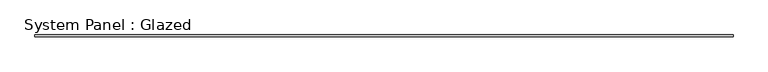
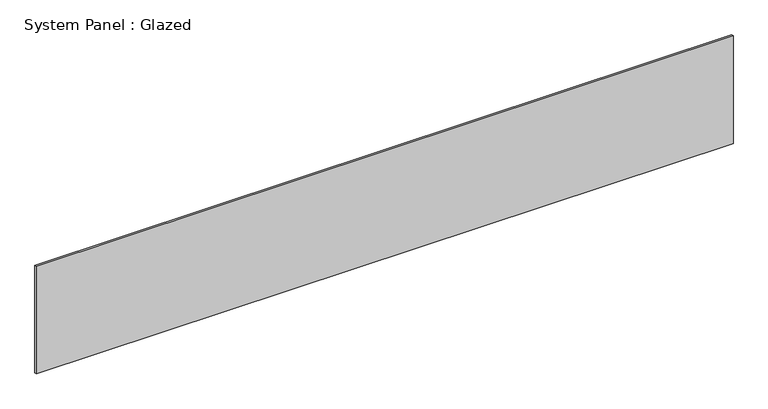
"""IFC4 building model written with IfcOpenShell, lengths in millimetres: plate geometry, System Panel : Glazed."""

from ifc_helpers import new_model, si_unit, origin, origin_with_axes, place, context, project, spatial, polyline, outline, extrude, source, transform, mapped, element, save


def system_panel_glazed_da9a879b(model_context):
    return source(origin(), model_context, "Body", "SweptSolid", [
        extrude(outline(polyline([(4670.425, 19.05), (-4670.425, 19.05), (-4670.425, 44.45), (4670.425, 44.45), (4670.425, 19.05)])), origin_with_axes(), (0.0, 0.0, 1.0), 1524.0),
    ])


if __name__ == "__main__":
    model = new_model("IFC4")
    model_context = context("Model", 3, world=origin())
    ifc_project = project(units=[si_unit("LENGTHUNIT", "METRE", prefix="MILLI")], contexts=[model_context])
    site = spatial("IfcSite", under=ifc_project)
    building = spatial("IfcBuilding", under=site)
    placement = place(None, origin())
    system_panel_glazed_shape = system_panel_glazed_da9a879b(model_context)
    element("IfcPlate", 1, ObjectType="System Panel : Glazed", at=placement, inside=building, context=model_context, shape_type="MappedRepresentation", body=[
        mapped(system_panel_glazed_shape, transform((0.0, 0.0, 0.0), x_axis=(1.0, 0.0, 0.0), y_axis=(0.0, 1.0, 0.0), z_axis=(0.0, 0.0, 1.0))),
    ])
    save(model, "model.ifc")

# Revit data of these elements
# Type "System Panel : Glazed"
#   Construction Type Id = "GSP4R"
#   Analytic Construction = "1/8 in Pilkington single glazing"
#   Visual Light Transmittance = 0.9
#   Solar Heat Gain Coefficient = 0.86
#   Heat Transfer Coefficient (U) = 1.18115 BTU/(h·ft²·°F)
# Element 1 (IfcPlate, "System Panel : Glazed")
#   Materials on its faces: "Glass"
# Materials
#   "Glass": class "Glass", colour RGB 0 128 192, transparency 0.75, Description = "Soda Lime Glass", Cost = 0
